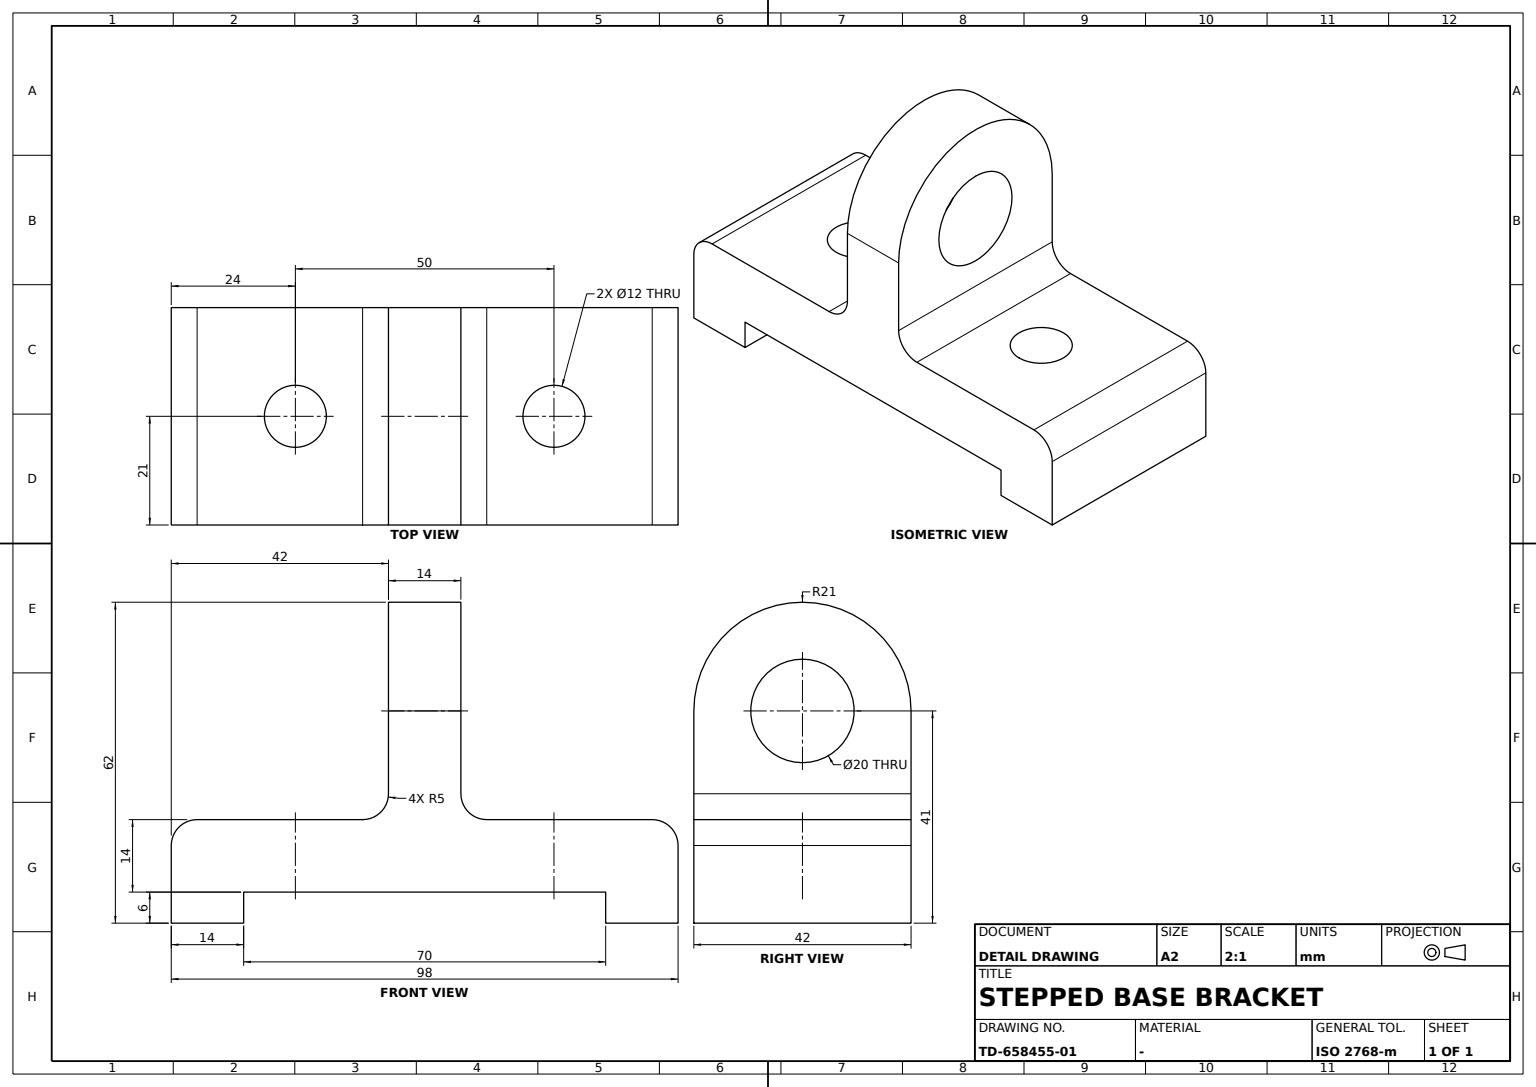
CATIA V5 part; units mm, degrees
sketch "Sketch1" plane through (0, 0, 0) normal (1, 0, 0) x (0, 1, 0)
  line L0 (-49, 7) -> (-49, -13)
  line L1 (-49, -13) -> (-35, -13)
  line L2 (-35, -13) -> (-35, -7)
  line L3 (-35, -7) -> (35, -7)
  line L4 (35, -7) -> (35, -13)
  point P0 (35, -13)
  line L5 (35, -13) -> (49, -13)
  line L6 (49, -13) -> (49, 7)
  line L7 (49, 7) -> (-49, 7)
  dimension "length L1" = 14
  dimension "length L3" = 70
  dimension "length L5" = 14
  dimension "length L0" = 20
  dimension "length L4" = 6
  constraint vertical L0 y-axis
  constraint vertical L2 y-axis
  constraint vertical L4 y-axis
  constraint vertical L6 y-axis
  constraint horizontal L1 x-axis
  constraint horizontal L3 x-axis
  constraint horizontal L5 x-axis
  constraint horizontal L7 x-axis
  constraint coincidence P0 L1
  constraint symmetry L0 L6 y-axis
  constraint symmetry L3 L7 x-axis
extrude "Pad1" add sketch "Sketch1" along normal mid plane 42
sketch "Sketch2" plane through (0, 0, 0) normal (0, 1, 0) x (-1, 0, 0)
  arc A0 (21, 28) -> (-21, 28) centre (0, 28) ccw
  point P0 (0, 28)
  circle A1 centre (0, 28) radius 10
  line L0 (-21, 28) -> (-21, 7)
  point P1 (-21, 7)
  line L1 (21, 28) -> (21, 7)
  point P2 (21, 7)
  line L2 (21, 7) -> (-21, 7) construction
  line L3 (21, 7) -> (-21, 7) construction
  line L4 (21, 7) -> (-21, 7) construction
  line L5 (21, 7) -> (-21, 7)
  dimension "radius A0" = 21
  dimension "radius A1" = 10
  dimension "distance P0 L4" = 21
  constraint coincidence P0 y-axis
  constraint coincidence P2 L2
  constraint coincidence P1 L3
  constraint vertical L0 y-axis
  constraint vertical L1 y-axis
  constraint tangency L1 A0
  constraint tangency L0 A0
extrude "Pad2" add sketch "Sketch2" along normal mid plane 14
sketch "Sketch3" plane through (0, 0, 7) normal (0, 0, 1) x (0, 1, 0)
  circle A0 centre (25, 0) radius 6
  point P0 (25, 0)
  line L0 (49, 21) -> (49, -21) construction
  circle A1 centre (-25, 0) radius 6
  dimension "radius A0" = 6
  dimension "distance P0 L0" = 24
  constraint coincidence P0 x-axis
  constraint symmetry A0 A1 y-axis
extrude "Pocket1" cut sketch "Sketch3" against normal up to next
fillet "Fillet1" radius 5 1 edges at (0, -49, 7)
fillet "Fillet2" radius 5 1 edges at (0, 49, 7)
fillet "Fillet3" radius 5 1 edges at (0, 7, 7)
fillet "Fillet4" radius 5 1 edges at (0, -7, 7)
